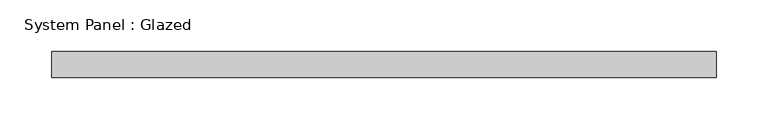
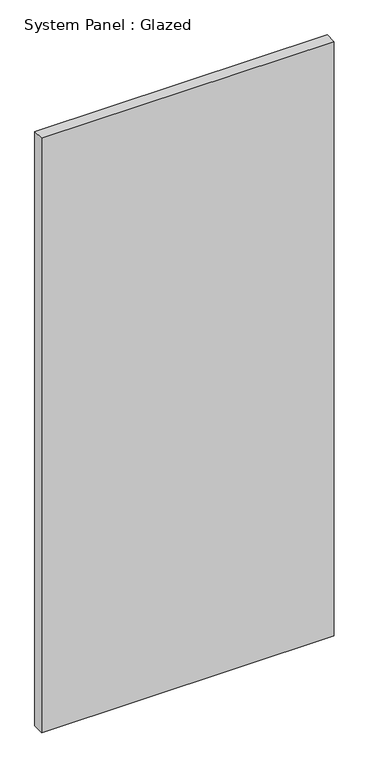
"""IFC4 building model written with IfcOpenShell, lengths in millimetres: plate geometry, System Panel : Glazed."""

from ifc_helpers import new_model, si_unit, origin, origin_with_axes, place, context, project, spatial, polyline, outline, extrude, source, transform, mapped, element, save


def system_panel_glazed_95f8db0f(model_context):
    return source(origin(), model_context, "Body", "SweptSolid", [
        extrude(outline(polyline([(322.7916667, 19.05), (-322.7916667, 19.05), (-322.7916667, 44.45), (322.7916667, 44.45), (322.7916667, 19.05)])), origin_with_axes(), (0.0, 0.0, 1.0), 1386.5761917),
    ])


if __name__ == "__main__":
    model = new_model("IFC4")
    model_context = context("Model", 3, world=origin())
    ifc_project = project(units=[si_unit("LENGTHUNIT", "METRE", prefix="MILLI")], contexts=[model_context])
    site = spatial("IfcSite", under=ifc_project)
    building = spatial("IfcBuilding", under=site)
    placement = place(None, origin())
    system_panel_glazed_shape = system_panel_glazed_95f8db0f(model_context)
    element("IfcPlate", 1, ObjectType="System Panel : Glazed", at=placement, inside=building, context=model_context, shape_type="MappedRepresentation", body=[
        mapped(system_panel_glazed_shape, transform((0.0, 0.0, 0.0), x_axis=(1.0, 0.0, 0.0), y_axis=(0.0, 1.0, 0.0), z_axis=(0.0, 0.0, 1.0))),
    ])
    save(model, "model.ifc")

# Revit data of these elements
# Type "System Panel : Glazed"
#   Construction Type Id = "GSP4R"
#   Analytic Construction = "1/8 in Pilkington single glazing"
#   Visual Light Transmittance = 0.9
#   Solar Heat Gain Coefficient = 0.86
#   Heat Transfer Coefficient (U) = 1.18115 BTU/(h·ft²·°F)
#   Define Thermal Properties by = 1
# Element 1 (IfcPlate, "System Panel : Glazed")
#   Materials on its faces: "Glass"
# Materials
#   "Glass": class "Glass", colour RGB 0 128 192, transparency 0.75, Description = "Soda Lime Glass", Cost = 0
